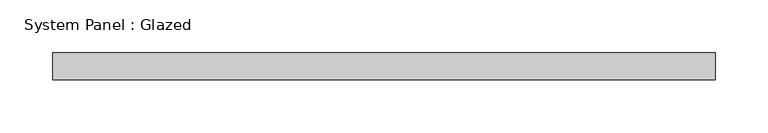
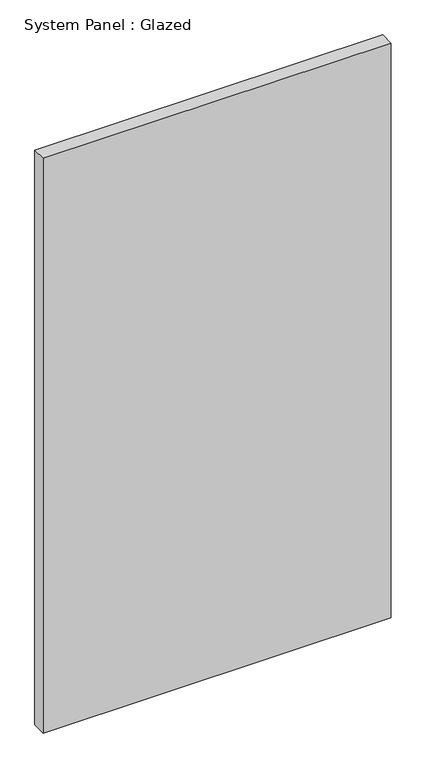
"""IFC4 building model written with IfcOpenShell, lengths in millimetres: plate geometry, System Panel : Glazed."""

from ifc_helpers import new_model, si_unit, origin, origin_with_axes, place, context, project, spatial, polyline, outline, extrude, source, transform, mapped, element, save


def system_panel_glazed_b9e36109(model_context):
    return source(origin(), model_context, "Body", "SweptSolid", [
        extrude(outline(polyline([(312.9206736, 19.05), (-312.9206736, 19.05), (-312.9206736, 44.45), (312.9206736, 44.45), (312.9206736, 19.05)])), origin_with_axes(), (0.0, 0.0, 1.0), 1092.2),
    ])


if __name__ == "__main__":
    model = new_model("IFC4")
    model_context = context("Model", 3, world=origin())
    ifc_project = project(units=[si_unit("LENGTHUNIT", "METRE", prefix="MILLI")], contexts=[model_context])
    site = spatial("IfcSite", under=ifc_project)
    building = spatial("IfcBuilding", under=site)
    placement = place(None, origin())
    system_panel_glazed_shape = system_panel_glazed_b9e36109(model_context)
    element("IfcPlate", 1, ObjectType="System Panel : Glazed", at=placement, inside=building, context=model_context, shape_type="MappedRepresentation", body=[
        mapped(system_panel_glazed_shape, transform((0.0, 0.0, 0.0), x_axis=(1.0, 0.0, 0.0), y_axis=(0.0, 1.0, 0.0), z_axis=(0.0, 0.0, 1.0))),
    ])
    save(model, "model.ifc")

# Revit data of these elements
# Type "System Panel : Glazed"
#   Construction Type Id = "GSP4R"
#   Analytic Construction = "1/8 in Pilkington single glazing"
#   Visual Light Transmittance = 0.9
#   Solar Heat Gain Coefficient = 0.86
#   Heat Transfer Coefficient (U) = 1.18115 BTU/(h·ft²·°F)
# Element 1 (IfcPlate, "System Panel : Glazed")
#   Materials on its faces: "Glass"
# Materials
#   "Glass": class "Glass", colour RGB 0 128 192, transparency 0.75, Description = "Soda Lime Glass", Cost = 0
